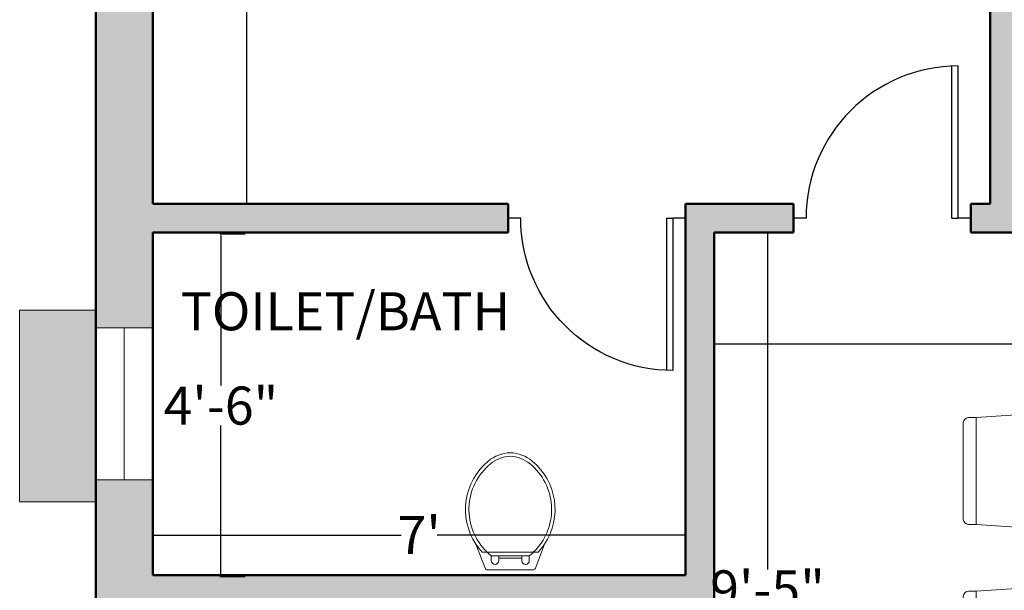
# Model space of a CAD drawing. Units: inches. Extents: x -28 to 544, y -640 to 52.
# Tile 6 of 11: x 5 to 160, y -194 to -104. Entities that reach past the tile are written whole.
import ezdxf

# ---------------------------------------------------------------- set-up
doc = ezdxf.new("R2010")
doc.units = ezdxf.units.IN
doc.header["$MEASUREMENT"] = 0
for name, color, linetype, lineweight in [('A-ANNO-DIMS', 2, 'Continuous', 18), ('A-AREA-IDEN', 7, 'Continuous', 25), ('A-DOOR', 3, 'Continuous', 25), ('A-FLOR-FIXT', 9, 'Continuous', 20), ('A-FURN', 8, 'Continuous', 18), ('A-GLAZ', 4, 'Continuous', 20), ('A-ROOF', 8, 'Continuous', 18), ('A-ROOF-PATT', 252, 'Continuous', 13), ('A-WALL', 7, 'Continuous', 50), ('A-WALL-PATT', 5, 'Continuous', 13)]:
    doc.layers.add(name, color=color, linetype=linetype, lineweight=lineweight)
doc.styles.get("Standard").update_dxf_attribs({"font": 'arial.ttf'})
doc.dimstyles.get("Standard").update_dxf_attribs({"dimtxt": 0.18, "dimasz": 0.18, "dimexe": 0.18, "dimexo": 0.0625, "dimgap": 0.09, "dimtad": 0, "dimtih": 1, "dimtoh": 1, "dimdec": 0, "dimzin": 0, "dimdsep": 46, "dimlunit": 3, "dimtxsty": 'Standard', "dimcen": 0.09, "dimadec": 0, "dimazin": 0, "dimtfac": 1, "dimtdec": 0, "dimtofl": 0, "dimtmove": 0, "dimatfit": 3, "dimfxl": 1, "dimtolj": 1, "dimtzin": 0, "dimarcsym": 0})

# ---------------------------------------------------------------- blocks, each defined once
blk = doc.blocks.new('*D1')
at = {"layer": 'A-ANNO-DIMS', "color": 0, "lineweight": -2, "transparency": 16777216}
for p, q in [((40.67, -1.24), (40.56, -1.24)), ((40.74, -1.42), (40.74, -64.14)), ((40.74, -133.06), (40.74, -70.34)), ((40.67, -133.24), (40.56, -133.24))]:
    blk.add_line(p, q, dxfattribs=at)
at = {"layer": 'A-ANNO-DIMS', "color": 0, "transparency": 16777216}
for points in [[(40.71, -1.42), (40.77, -1.42), (40.74, -1.24)], [(40.71, -133.06), (40.77, -133.06), (40.74, -133.24)]]:
    blk.add_solid(points, dxfattribs=at)
at = {"layer": 'Defpoints', "color": 0, "transparency": 16777216}
for p in [(40.74, -1.24), (40.74, -133.24), (40.74, -133.24)]:
    blk.add_point(p, dxfattribs=at)
at = {"layer": 'A-ANNO-DIMS', "color": 0, "transparency": 16777216, "insert": (40.74, -67.24), "char_height": 6, "attachment_point": 5}
blk.add_mtext("\\A1;11'", dxfattribs=at)
blk = doc.blocks.new('*D9')
at = {"layer": 'A-ANNO-DIMS', "color": 0, "lineweight": -2, "transparency": 16777216}
for p, q in [((40.5, -138.02), (36.49, -138.02)), ((36.67, -138.2), (36.67, -161.87)), ((36.67, -191.84), (36.67, -168.17)), ((40.5, -192.02), (36.49, -192.02))]:
    blk.add_line(p, q, dxfattribs=at)
at = {"layer": 'A-ANNO-DIMS', "color": 0, "transparency": 16777216}
for points in [[(36.64, -138.2), (36.7, -138.2), (36.67, -138.02)], [(36.64, -191.84), (36.7, -191.84), (36.67, -192.02)]]:
    blk.add_solid(points, dxfattribs=at)
at = {"layer": 'Defpoints', "color": 0, "transparency": 16777216}
for p in [(40.56, -138.02), (36.67, -192.02), (40.56, -192.02)]:
    blk.add_point(p, dxfattribs=at)
at = {"layer": 'A-ANNO-DIMS', "color": 0, "transparency": 16777216, "insert": (36.67, -165.02), "char_height": 6, "attachment_point": 5}
blk.add_mtext('\\A1;4\'-6"', dxfattribs=at)
blk = doc.blocks.new('*D10')
at = {"layer": 'A-ANNO-DIMS', "color": 0, "lineweight": -2, "transparency": 16777216}
for p, q in [((25.94, -182.71), (25.94, -185.6)), ((26.12, -185.42), (65.12, -185.42)), ((109.76, -185.42), (70.77, -185.42)), ((109.94, -185.36), (109.94, -185.24))]:
    blk.add_line(p, q, dxfattribs=at)
at = {"layer": 'A-ANNO-DIMS', "color": 0, "transparency": 16777216}
for points in [[(26.12, -185.39), (26.12, -185.45), (25.94, -185.42)], [(109.76, -185.39), (109.76, -185.45), (109.94, -185.42)]]:
    blk.add_solid(points, dxfattribs=at)
at = {"layer": 'Defpoints', "color": 0, "transparency": 16777216}
for p in [(25.94, -182.65), (109.94, -185.42), (109.94, -185.42)]:
    blk.add_point(p, dxfattribs=at)
at = {"layer": 'A-ANNO-DIMS', "color": 0, "transparency": 16777216, "insert": (67.94, -185.42), "char_height": 6, "attachment_point": 5}
blk.add_mtext("\\A1;7'", dxfattribs=at)
blk = doc.blocks.new('*D35')
at = {"layer": 'A-ANNO-DIMS', "color": 0, "lineweight": -2, "transparency": 16777216}
for p, q in [((126.88, -137.74), (122.68, -137.74)), ((122.86, -137.92), (122.86, -190.84)), ((122.86, -250.06), (122.86, -197.14)), ((127.88, -250.24), (122.68, -250.24))]:
    blk.add_line(p, q, dxfattribs=at)
at = {"layer": 'A-ANNO-DIMS', "color": 0, "transparency": 16777216}
for points in [[(122.83, -137.92), (122.89, -137.92), (122.86, -137.74)], [(122.83, -250.06), (122.89, -250.06), (122.86, -250.24)]]:
    blk.add_solid(points, dxfattribs=at)
at = {"layer": 'Defpoints', "color": 0, "transparency": 16777216}
for p in [(126.94, -137.74), (122.86, -250.24), (127.94, -250.24)]:
    blk.add_point(p, dxfattribs=at)
at = {"layer": 'A-ANNO-DIMS', "color": 0, "transparency": 16777216, "insert": (122.86, -193.99), "char_height": 6, "attachment_point": 5}
blk.add_mtext('\\A1;9\'-5"', dxfattribs=at)
blk = doc.blocks.new('*D37')
at = {"layer": 'A-ANNO-DIMS', "color": 0, "lineweight": -2, "transparency": 16777216}
for p, q in [((114.44, -152.03), (114.44, -155.48)), ((246.44, -152.03), (246.44, -155.48)), ((114.62, -155.3), (175.55, -155.3)), ((246.26, -155.3), (185.34, -155.3))]:
    blk.add_line(p, q, dxfattribs=at)
at = {"layer": 'A-ANNO-DIMS', "color": 0, "transparency": 16777216}
for points in [[(114.62, -155.27), (114.62, -155.33), (114.44, -155.3)], [(246.26, -155.27), (246.26, -155.33), (246.44, -155.3)]]:
    blk.add_solid(points, dxfattribs=at)
at = {"layer": 'Defpoints', "color": 0, "transparency": 16777216}
for p in [(114.44, -151.97), (246.44, -151.97), (246.44, -155.3)]:
    blk.add_point(p, dxfattribs=at)
at = {"layer": 'A-ANNO-DIMS', "color": 0, "transparency": 16777216, "insert": (180.44, -155.3), "char_height": 6, "attachment_point": 5}
blk.add_mtext("\\A1;11'", dxfattribs=at)
blk = doc.blocks.new('DINING-SET-4')
for p, q in [((18.79, 50.59), (2.05, 49.45)), ((58.27, 50.59), (75.01, 49.45)), ((0, 33.45), (0, 48.63)), ((0.82, 49.45), (2.05, 49.45)), ((2.05, 32.63), (2.05, 49.45)), ((20.52, 48.95), (20.52, 33.13)), ((56.54, 48.95), (56.54, 33.13)), ((76.24, 49.45), (75.01, 49.45)), ((75.01, 32.63), (75.01, 49.45)), ((77.06, 33.45), (77.06, 48.63)), ((2.05, 32.63), (0.82, 32.63)), ((2.05, 32.63), (18.79, 31.49)), ((75.01, 32.63), (58.27, 31.49)), ((75.01, 32.63), (76.24, 32.63)), ((2.05, 22.09), (0.82, 22.09)), ((2.05, 22.09), (18.79, 23.23)), ((2.05, 22.09), (2.05, 5.27)), ((75.01, 22.09), (58.27, 23.23)), ((75.01, 22.09), (76.24, 22.09)), ((75.01, 22.09), (75.01, 5.27)), ((0, 21.27), (0, 6.09)), ((20.52, 5.77), (20.52, 21.59)), ((56.54, 5.77), (56.54, 21.59)), ((77.06, 21.27), (77.06, 6.09)), ((0.82, 5.27), (2.05, 5.27)), ((18.79, 4.13), (2.05, 5.27)), ((58.27, 4.13), (75.01, 5.27)), ((76.24, 5.27), (75.01, 5.27))]:
    blk.add_line(p, q)
for points in [[(55.63, 0), (21.43, 0), (21.43, 54.72), (55.63, 54.72)], [(53.35, 2.28), (23.71, 2.28), (23.71, 52.44), (53.35, 52.44)]]:
    blk.add_lwpolyline(points, close=True)
for centre, radius, start, end in [((18.88, 48.95), 1.64, 0, 93.1221), ((58.18, 48.95), 1.64, 86.8779, 180), ((0.82, 48.63), 0.821, 90, 180), ((76.24, 48.63), 0.821, 0, 90), ((0.82, 33.45), 0.821, 180, 270), ((18.88, 33.13), 1.64, 266.8779, 0), ((58.18, 33.13), 1.64, 180, 273.1221), ((76.24, 33.45), 0.821, 270, 0), ((0.82, 21.27), 0.821, 90, 180), ((18.88, 21.59), 1.64, 0, 93.1221), ((58.18, 21.59), 1.64, 86.8779, 180), ((76.24, 21.27), 0.821, 0, 90), ((0.82, 6.09), 0.821, 180, 270), ((18.88, 5.77), 1.64, 266.8779, 0), ((58.18, 5.77), 1.64, 180, 273.1221), ((76.24, 6.09), 0.821, 270, 0)]:
    blk.add_arc(centre, radius, start, end)
blk = doc.blocks.new('WC-PLAN')
for p, q in [((3.43, 2.8), (2.65, 2.8)), ((3.43, 2.8), (7.07, 2.8)), ((10.7, 2.8), (7.07, 2.8)), ((11.48, 2.8), (10.7, 2.8))]:
    blk.add_line(p, q)
for points in [[(1.65, 4.07, -0.383919), (3.59, 17.16, -0.163732), (7.07, 18.49, -0.359733)], [(3.43, 2.8, -0.448546), (3.94, 16.74, -0.162618), (7.07, 17.94, -0.470877)], [(12.48, 4.07, 0.383919), (10.54, 17.16, 0.163732), (7.07, 18.49, 0.359733)], [(11.08, 3.18, 0.431639), (10.19, 16.74, 0.162618), (7.07, 17.94, 0.470877)], [(2.65, 2.8, -0.040937), (1.65, 4.07, -0.163732)], [(7.07, 0), (3.53, 0, -0.31031), (3.1, 0.3), (1.65, 4.07, -0.209071)], [(7.07, 0), (10.6, 0, 0.31031), (11.03, 0.3), (12.48, 4.07, 0.209071)], [(10.7, 2.8, 0.014165), (11.08, 3.18, 0.162618)], [(11.48, 2.8, 0.040937), (12.48, 4.07, 0.163732)], [(4.07, 2.24, -0.022712), (3.43, 2.8, -0.162618)], [(7.07, 2.24), (4.07, 2.24, -0.476108)], [(4.07, 2.24), (4.07, 1.47, 1), (5.25, 1.47), (5.25, 1.87)], [(7.07, 2.24), (10.07, 2.24, 0.022712)], [(10.07, 2.24), (10.07, 1.47, -1), (8.89, 1.47), (8.89, 1.87)], [(10.07, 2.24, 0.022712), (10.7, 2.8, 0.162618)]]:
    blk.add_lwpolyline(points, format="xyb")
for points in [[(5.25, 1.87), (5.25, 2.24)], [(5.25, 1.87), (8.89, 1.87)], [(8.89, 1.87), (8.89, 2.24)]]:
    blk.add_lwpolyline(points)
blk = doc.blocks.new('WIN-24IN')
for p, q in [((0, 0), (0, 24)), ((0, 24), (9, 24)), ((4.5, 0), (4.5, 24)), ((9, 24), (9, 0)), ((9, 0), (0, 0))]:
    blk.add_line(p, q)
blk = doc.blocks.new('DOOR-SWING-24IN')
for p, q in [((25, 0), (25, 24)), ((26, 0), (26, 24)), ((2, 0), (0, 0)), ((25, 0), (26, 0)), ((28, 0), (26, 0))]:
    blk.add_line(p, q)
blk.add_arc((26, 0), 24, 90, 180)

msp = doc.modelspace()

# ---------------------------------------------------------------- hatches: boundary and pattern name
at = {"layer": 'A-ROOF-PATT'}
h = msp.add_hatch(color=256, dxfattribs=at)
h.dxf.hatch_style = 1
h.set_gradient(color1=(241, 235, 31), color2=(248, 153, 30))
h.paths.add_polyline_path([(124.53, 19.76), (58.75, 19.76), (58.75, 7.76), (124.53, 7.76)])
h.paths.add_polyline_path([(226.33, 19.76), (182.83, 19.76), (182.83, 7.76), (226.33, 7.76)])
h.paths.add_polyline_path([(313.67, 19.76), (271.84, 19.76), (271.84, 7.76), (313.67, 7.76)])
h.paths.add_polyline_path([(440.55, 19.76), (372.16, 19.76), (372.16, 7.76), (440.55, 7.76)])
h.paths.add_polyline_path([(492.44, -34.91), (480.44, -34.91), (480.44, -100.18), (492.44, -100.18)])
h.paths.add_polyline_path([(492.44, -151.37), (480.44, -151.37), (480.44, -179.02), (492.44, -179.02)])
h.paths.add_polyline_path([(492.44, -207.96), (480.44, -207.96), (480.44, -238.77), (492.44, -238.77)])
h.paths.add_polyline_path([(492.44, -289.99), (480.44, -289.99), (480.44, -354.53), (492.44, -354.53)])
h.paths.add_polyline_path([(492.44, -399.27), (480.44, -399.27), (480.44, -430), (492.44, -430)])
h.paths.add_polyline_path([(492.44, -475.99), (480.44, -475.99), (480.44, -546.14), (492.44, -546.14)])
h.paths.add_polyline_path([(442.7, -587.74), (368.43, -587.74), (368.43, -599.74), (442.7, -599.74)])
h.paths.add_polyline_path([(127.64, -587.74), (54.75, -587.74), (54.75, -599.74), (127.64, -599.74)])
h.paths.add_polyline_path([(16.94, -477.43), (4.94, -477.43), (4.94, -547.54), (16.94, -547.54)])
h.paths.add_polyline_path([(16.94, -399.8), (4.94, -399.8), (4.94, -430.58), (16.94, -430.58)])
h.paths.add_polyline_path([(16.94, -287.93), (4.94, -287.93), (4.94, -356.82), (16.94, -356.82)])
h.paths.add_polyline_path([(16.94, -208.93), (4.94, -208.93), (4.94, -240.18), (16.94, -240.18)])
h.paths.add_polyline_path([(16.94, -150), (4.94, -150), (4.94, -180.17), (16.94, -180.17)])
h.paths.add_polyline_path([(16.94, -32.89), (4.94, -32.89), (4.94, -101.73), (16.94, -101.73)])
at = {"layer": 'A-WALL-PATT'}
h = msp.add_hatch(color=256, dxfattribs=at)
h.dxf.hatch_style = 1
h.paths.add_polyline_path([(25.94, -235.24), (16.94, -235.24), (16.94, -290.74), (25.94, -290.74), (25.94, -254.74), (127.94, -254.74), (127.94, -252.49), (127.94, -250.24), (118.94, -250.24), (118.94, -247.24), (109.94, -247.24), (109.94, -250.24), (25.94, -250.24)])
h.paths.add_polyline_path([(114.44, -191.74), (114.44, -137.74), (126.94, -137.74), (126.94, -135.49), (126.94, -133.24), (109.94, -133.24), (109.94, -137.74), (109.94, -191.74), (25.94, -191.74), (25.94, -176.74), (16.94, -176.74), (16.94, -211.24), (25.94, -211.24), (25.94, -196.24), (109.94, -196.24), (109.94, -219.24), (114.44, -219.24), (114.44, -196.24)])
h.paths.add_polyline_path([(25.94, -350.74), (16.94, -350.74), (16.94, -403.24), (25.94, -403.24), (25.94, -391.24), (121.94, -391.24), (121.94, -403.24), (126.44, -403.24), (126.44, -391.24), (162.44, -391.24), (162.44, -250.24), (155.94, -250.24), (155.94, -254.74), (157.94, -254.74), (157.94, -386.74), (25.94, -386.74)])
h.paths.add_polyline_path([(25.94, -443.74), (157.94, -443.74), (157.94, -446.74), (162.44, -446.74), (162.44, -439.24), (126.44, -439.24), (126.44, -427.74), (121.94, -427.74), (121.94, -439.24), (25.94, -439.24), (25.94, -427.24), (16.94, -427.24), (16.94, -481.24), (25.94, -481.24)])
h.paths.add_polyline_path([(25.94, -541.24), (16.94, -541.24), (16.94, -587.74), (61.94, -587.74), (61.94, -578.74), (25.94, -578.74)])
h.paths.add_polyline_path([(162.44, -578.74), (162.44, -474.74), (160.19, -474.74), (157.94, -474.74), (157.94, -578.74), (121.94, -578.74), (121.94, -587.74), (162.44, -587.74)])
h.paths.add_polyline_path([(200.69, -578.74), (162.44, -578.74), (162.44, -587.74), (200.69, -587.74)])
h.paths.add_polyline_path([(25.94, -97.24), (16.94, -97.24), (16.94, -152.74), (25.94, -152.74), (25.94, -137.74), (81.94, -137.74), (81.94, -135.49), (81.94, -133.24), (25.94, -133.24)])
h.paths.add_polyline_path([(210.44, -133.24), (162.44, -133.24), (162.44, -1.24), (186.44, -1.24), (186.44, 7.76), (121.94, 7.76), (121.94, -1.24), (157.94, -1.24), (157.94, -133.24), (154.94, -133.24), (154.94, -137.74), (210.44, -137.74)])
h.paths.add_polyline_path([(61.94, 7.76), (16.94, 7.76), (16.94, -37.24), (25.94, -37.24), (25.94, -1.24), (61.94, -1.24)])

# ---------------------------------------------------------------- linework, layer by layer
at = {"layer": 'A-ROOF'}
for p, q in [((4.94, -180.17), (4.94, -150)), ((4.94, -150), (16.94, -150)), ((16.94, -180.17), (4.94, -180.17))]:
    msp.add_line(p, q, dxfattribs=at)
at = {"layer": 'A-WALL'}
for p, q in [((16.94, 7.76), (16.94, -587.74)), ((25.94, -1.24), (25.94, -133.24)), ((157.94, -1.24), (157.94, -133.24)), ((25.94, -133.24), (81.94, -133.24)), ((81.94, -135.49), (81.94, -133.24)), ((109.94, -137.74), (109.94, -133.24)), ((109.94, -133.24), (126.94, -133.24)), ((126.94, -135.49), (126.94, -133.24)), ((154.94, -133.24), (154.94, -137.74)), ((154.94, -133.24), (157.94, -133.24)), ((81.94, -135.49), (81.94, -137.74)), ((126.94, -135.49), (126.94, -137.74)), ((25.94, -137.74), (81.94, -137.74)), ((25.94, -137.74), (25.94, -191.74)), ((109.94, -137.74), (109.94, -191.74)), ((114.44, -137.74), (126.94, -137.74)), ((114.44, -137.74), (114.44, -191.74)), ((154.94, -137.74), (210.44, -137.74)), ((25.94, -191.74), (109.94, -191.74)), ((114.44, -191.74), (114.44, -196.24))]:
    msp.add_line(p, q, dxfattribs=at)

# ---------------------------------------------------------------- block references
at = {"layer": 'A-DOOR'}
msp.add_blockref('DOOR-SWING-24IN', (126.94, -135.49), dxfattribs=at)
at = {"layer": 'A-DOOR', "extrusion": (0, 0, -1), "zscale": -1, "rotation": 180}
msp.add_blockref('DOOR-SWING-24IN', (-81.95, -135.49), dxfattribs=at)
at = {"layer": 'A-FLOR-FIXT'}
msp.add_blockref('WC-PLAN', (75.23, -190.93), dxfattribs=at)
at = {"layer": 'A-FURN'}
msp.add_blockref('DINING-SET-4', (153.73, -216.37), dxfattribs=at)
at = {"layer": 'A-GLAZ', "rotation": 180}
msp.add_blockref('WIN-24IN', (25.94, -152.74), dxfattribs=at)

# ---------------------------------------------------------------- texts
at = {"layer": 'A-AREA-IDEN', "insert": (30.34, -147.15), "char_height": 6, "attachment_point": 1}
msp.add_mtext('TOILET/BATH', dxfattribs=at)

# ---------------------------------------------------------------- dimensions: what is measured, and where the dimension line sits
at = {"layer": 'A-ANNO-DIMS'}
for base, p1, p2, picture, middle in [((40.74, -133.24), (40.74, -1.24), (40.74, -133.24), '*D1', (40.74, -67.24)), ((36.67, -192.02), (40.56, -138.02), (40.56, -192.02), '*D9', (36.67, -165.02)), ((122.8647962, -250.24117838), (126.94473605, -137.74117838), (127.94473605, -250.24117838), '*D35', (122.8647962, -193.99117838))]:
    dim = msp.add_linear_dim(base=base, p1=p1, p2=p2, angle=90, dimstyle='Standard', override={"dimtxt": 6, "dimclrd": 0, "dimclre": 0, "dimclrt": 0}, dxfattribs=at)
    dim.commit()
    dim.dimension.update_dxf_attribs({"geometry": picture, "text_midpoint": middle})
for base, p1, p2, picture, middle in [((246.44, -155.3), (114.44, -151.97), (246.44, -151.97), '*D37', (180.44, -155.3)), ((109.94, -185.42), (25.94, -182.65), (109.94, -185.42), '*D10', (67.94, -185.42))]:
    dim = msp.add_linear_dim(base=base, p1=p1, p2=p2, dimstyle='Standard', override={"dimtxt": 6, "dimclrd": 0, "dimclre": 0, "dimclrt": 0}, dxfattribs=at)
    dim.commit()
    dim.dimension.update_dxf_attribs({"geometry": picture, "text_midpoint": middle})

doc.saveas('drawing.dxf')
